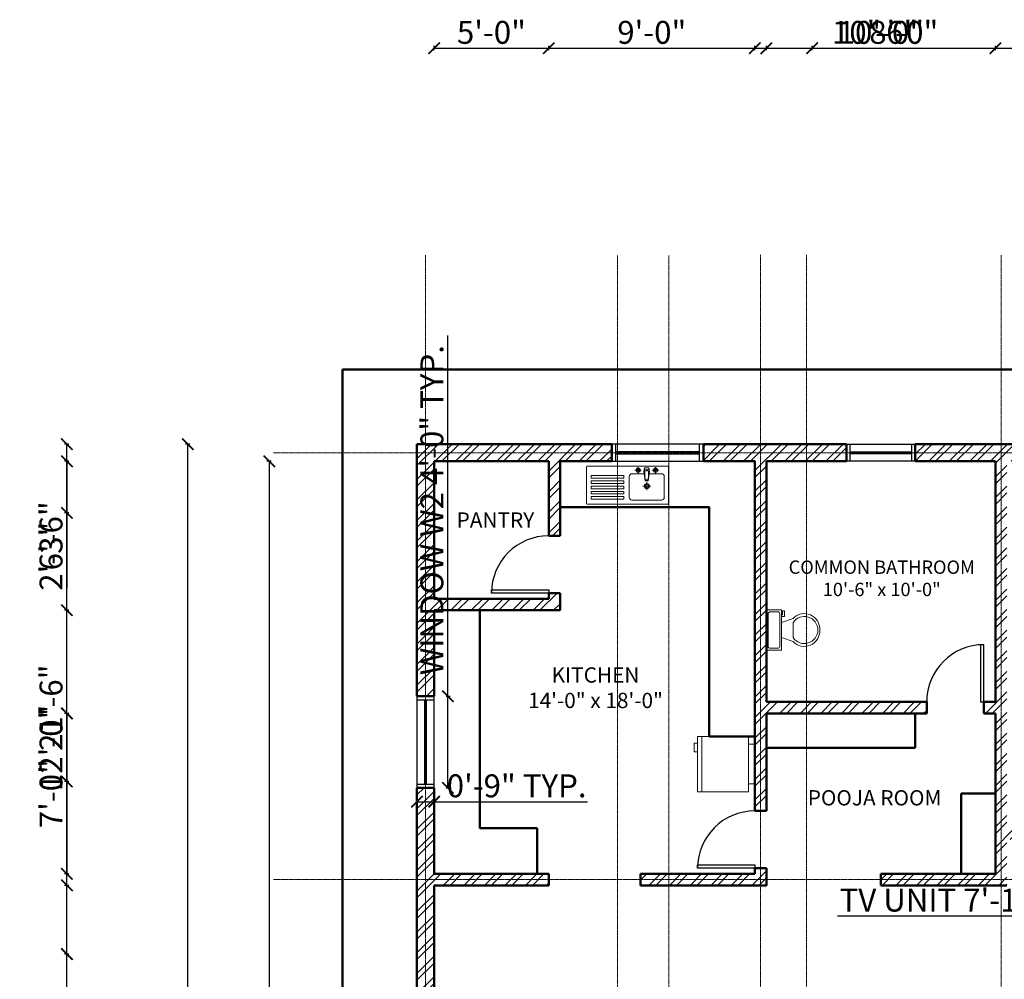
# Model space of a CAD drawing. Units: inches. Extents: x 261 to 2725, y 291 to 1454.
# Tile 13 of 35: x 261 to 777, y 951 to 1454. Entities that reach past the tile are written whole.
import ezdxf

# ---------------------------------------------------------------- set-up
doc = ezdxf.new("R2010")
doc.units = ezdxf.units.IN
doc.linetypes.add('CENTER', pattern=[2, 1.25, -0.25, 0.25, -0.25])
for name, color, linetype, lineweight in [('A-ANNO-DIMS', 136, 'Continuous', 18), ('A-AREA-IDEN', 18, 'Continuous', 18), ('A-DOOR', 160, 'Continuous', 25), ('A-FLOR-FIXT', 145, 'Continuous', 18), ('A-GLAZ', 150, 'Continuous', 25), ('A-GRID', 251, 'CENTER', 13), ('A-WALL', 222, 'Continuous', 50), ('A-WALL-PATT', 243, 'Continuous', 13)]:
    doc.layers.add(name, color=color, linetype=linetype, lineweight=lineweight)
doc.styles.get("Standard").update_dxf_attribs({"font": 'arial.ttf'})
doc.dimstyles.new('ISO-25', dxfattribs={"dimtxt": 12, "dimasz": 6, "dimexe": 1.25, "dimexo": 0.625, "dimtad": 1, "dimdec": 0, "dimlunit": 3, "dimtxsty": 'Standard', "dimblk": 'ARCHTICK', "dimcen": 2.5, "dimadec": 0, "dimazin": 0, "dimtfac": 1, "dimtdec": 0, "dimtmove": 0, "dimatfit": 3, "dimfxl": 1, "dimfxlon": 1, "dimarcsym": 0})

# ---------------------------------------------------------------- blocks, each defined once
blk = doc.blocks.new('*U3')
for p, q in [((0, 0), (0, -6)), ((30, 0), (30, -6))]:
    blk.add_line(p, q)
blk.add_lwpolyline([(0, 0), (0, 30), (1.75, 30), (1.75, 0)], close=True)
blk.add_arc((0, 0), 30, 0, 90)
blk = doc.blocks.new('*U4')
for p, q in [((-30, 0), (-30, -6)), ((0, 0), (0, -6))]:
    blk.add_line(p, q)
blk.add_lwpolyline([(0, 0), (0, 30), (-1.75, 30), (-1.75, 0)], close=True)
blk.add_arc((0, 0), 30, 90, 180)
blk = doc.blocks.new('A$C7C492201')
for p, q in [((0, 10), (0, 427)), ((10, 437), (927, 437)), ((221, 349), (78, 349)), ((112, 389), (185, 389)), ((148, 425), (148, 352)), ((223, 415), (217, 376)), ((217, 376), (232, 268)), ((223, 415), (232, 268)), ((223, 415), (248, 415)), ((225, 395), (248, 395)), ((273, 415), (248, 415)), ((272, 395), (248, 395)), ((273, 415), (265, 268)), ((280, 376), (265, 268)), ((273, 415), (280, 376)), ((418, 349), (276, 349)), ((312, 389), (385, 389)), ((348, 425), (348, 352)), ((937, 10), (937, 427)), ((48, 319), (48, 79)), ((231, 279), (248, 279)), ((232, 268), (248, 268)), ((266, 279), (248, 279)), ((265, 268), (248, 268)), ((248, 253), (248, 163)), ((448, 319), (448, 79)), ((509, 328), (509, 298)), ((509, 328), (885, 328)), ((509, 298), (885, 298)), ((509, 268), (509, 238)), ((509, 268), (885, 268)), ((509, 238), (885, 238)), ((885, 328), (885, 298)), ((885, 268), (885, 238)), ((203, 208), (294, 208)), ((509, 208), (885, 208)), ((509, 208), (509, 178)), ((509, 178), (885, 178)), ((509, 148), (509, 118)), ((509, 148), (885, 148)), ((509, 118), (885, 118)), ((885, 208), (885, 178)), ((885, 148), (885, 118)), ((927, 0), (10, 0)), ((418, 49), (78, 49)), ((509, 88), (509, 58)), ((509, 88), (885, 88)), ((509, 58), (885, 58)), ((885, 88), (885, 58))]:
    blk.add_line(p, q)
for centre, radius in [((148, 389), 25), ((148, 389), 15), ((348, 389), 25), ((348, 389), 15), ((248, 208), 30), ((248, 208), 20)]:
    blk.add_circle(centre, radius)
for centre, radius, start, end in [((10, 427), 10, 90, 180), ((78, 319), 30, 90, 180), ((247, 388), 7.19, 80.5252, 279.4748), ((250, 388), 7.19, 260.5252, 99.4748), ((418, 319), 30, 0, 90), ((927, 427), 10, 0, 90), ((10, 10), 10, 180, 270), ((78, 79), 30, 180, 270), ((418, 79), 30, 270, 0), ((927, 10), 10, 270, 0)]:
    blk.add_arc(centre, radius, start, end)
blk = doc.blocks.new('A$C659B0DF6')
for p, q in [((423, 642), (423, 606)), ((513, 642), (423, 642)), ((513, 606), (513, 642)), ((585, 606), (0, 606)), ((0, 66), (0, 606)), ((585, 561), (0, 561)), ((585, 66), (585, 606)), ((0, 66), (585, 66)), ((82, 0), (82, 66)), ((503, 0), (503, 66)), ((82, 0), (503, 0))]:
    blk.add_line(p, q)
blk = doc.blocks.new('*U27')
for p, q in [((9.5, -6), (9.5, -2)), ((-10, -8.5), (-8, -8.5)), ((-10, -9.5), (-10, -8.5)), ((-7, -9.5), (-10, -9.5)), ((-8, -8.5), (-8, -8)), ((-7, -8), (-7, -9.5)), ((-4, -8), (-6, -14)), ((4, -8), (6, -14)), ((4, -14), (-4, -14))]:
    blk.add_line(p, q)
blk.add_lwpolyline([(10.5, -8), (10.5, 0), (-10.5, 0), (-10.5, -8)], close=True)
for points in [[(-9.5, -2), (-9.5, -6)], [(8.5, -1), (-8.5, -1)], [(-8.5, -7), (8.5, -7)]]:
    blk.add_lwpolyline(points)
for centre, radius, start, end in [((-8.625, -1.875), 0.8839, 81.8699, 188.1301), ((8.625, -1.875), 0.8839, 351.8699, 98.1301), ((-8.625, -6.125), 0.8839, 171.869898, 278.1301), ((8.625, -6.125), 0.8839, 261.8699, 8.1301), ((-0.4772, -19.9188), 8.0953, 133.01722, 273.38), ((0.0374, -19.8731), 7.127, 124.50543, 269.7), ((-0.0373, -19.8731), 7.127, 270.3, 55.4946), ((0.4773, -19.9188), 8.0953, 266.62, 46.9828)]:
    blk.add_arc(centre, radius, start, end)
blk = doc.blocks.new('_ArchTick')
at = {"color": 0, "linetype": 'ByBlock', "const_width": 0.15}
blk.add_lwpolyline([(-0.5, -0.5), (0.5, 0.5)], dxfattribs=at)
blk = doc.blocks.new('*D29')
at = {"layer": 'A-ANNO-DIMS', "color": 0, "lineweight": -2, "transparency": 16777216}
for p, q in [((350.37, 1231.47), (348.12, 1231.47)), ((349.37, 508.47), (349.37, 1231.47)), ((350.37, 508.47), (348.12, 508.47))]:
    blk.add_line(p, q, dxfattribs=at)
at = {"layer": 'Defpoints', "color": 0, "transparency": 16777216}
for p in [(349.37, 1231.47), (469.45, 1231.47), (469.45, 508.47)]:
    blk.add_point(p, dxfattribs=at)
at = {"layer": 'A-ANNO-DIMS', "color": 0, "lineweight": -2, "transparency": 16777216, "xscale": 6, "yscale": 6, "zscale": 6}
for p, rotation in [((349.37, 1231.47), 90), ((349.37, 508.47), 270)]:
    blk.add_blockref('_ArchTick', p, dxfattribs=dict(at, rotation=rotation))
at = {"layer": 'A-ANNO-DIMS', "color": 0, "transparency": 16777216, "insert": (342.61, 869.97), "char_height": 12, "attachment_point": 5, "rotation": 90}
blk.add_mtext('60\'-3"', dxfattribs=at)
blk = doc.blocks.new('*D30')
at = {"layer": 'A-ANNO-DIMS', "color": 0, "lineweight": -2, "transparency": 16777216}
for p, q in [((393.09, 1222.47), (390.84, 1222.47)), ((392.09, 1222.47), (392.09, 517.47)), ((393.09, 517.47), (390.84, 517.47))]:
    blk.add_line(p, q, dxfattribs=at)
at = {"layer": 'Defpoints', "color": 0, "transparency": 16777216}
for p in [(478.45, 1222.47), (392.09, 517.47), (478.45, 517.47)]:
    blk.add_point(p, dxfattribs=at)
at = {"layer": 'A-ANNO-DIMS', "color": 0, "lineweight": -2, "transparency": 16777216, "xscale": 6, "yscale": 6, "zscale": 6}
for p, rotation in [((392.09, 1222.47), 90), ((392.09, 517.47), 270)]:
    blk.add_blockref('_ArchTick', p, dxfattribs=dict(at, rotation=rotation))
at = {"layer": 'A-ANNO-DIMS', "color": 0, "transparency": 16777216, "insert": (385.34, 869.97), "char_height": 12, "attachment_point": 5, "rotation": 90}
blk.add_mtext('58\'-9"', dxfattribs=at)
blk = doc.blocks.new('WIN-48')
for p, q in [((478.45, 1097.47), (469.45, 1097.47)), ((473.45, 1097.47), (473.45, 1053.47)), ((474.45, 1053.47), (474.45, 1097.47)), ((469.45, 1053.47), (478.45, 1053.47))]:
    blk.add_line(p, q)
blk.add_lwpolyline([(478.45, 1099.47), (469.45, 1099.47), (469.45, 1051.47), (478.45, 1051.47)], close=True)
blk = doc.blocks.new('WIN-36')
for p, q in [((1252.08, 755.47), (1243.08, 755.47)), ((1247.08, 755.47), (1247.08, 723.47)), ((1248.08, 723.47), (1248.08, 755.47)), ((1243.08, 723.47), (1252.08, 723.47))]:
    blk.add_line(p, q)
blk.add_lwpolyline([(1252.08, 721.47), (1252.08, 757.47), (1243.08, 757.47), (1243.08, 721.47)], close=True)
blk = doc.blocks.new('*D47')
at = {"layer": 'A-ANNO-DIMS', "color": 0, "lineweight": -2, "ltscale": 0.07, "transparency": 16777216}
for p, q in [((836.24, 985.34), (836.24, 983.09)), ((931.53, 985.34), (931.53, 983.09)), ((836.24, 984.34), (689.66, 984.34)), ((931.53, 984.34), (836.24, 984.34))]:
    blk.add_line(p, q, dxfattribs=at)
at = {"layer": 'Defpoints', "color": 0, "ltscale": 0.07, "transparency": 16777216}
for p in [(836.24, 998.63), (931.53, 998.63), (836.24, 984.34)]:
    blk.add_point(p, dxfattribs=at)
at = {"layer": 'A-ANNO-DIMS', "color": 0, "lineweight": -2, "ltscale": 0.07, "transparency": 16777216, "xscale": 6, "yscale": 6, "zscale": 6, "rotation": 180}
blk.add_blockref('_ArchTick', (836.24, 984.34), dxfattribs=at)
at = {"layer": 'A-ANNO-DIMS', "color": 0, "lineweight": -2, "ltscale": 0.07, "transparency": 16777216, "xscale": 6, "yscale": 6, "zscale": 6}
blk.add_blockref('_ArchTick', (931.53, 984.34), dxfattribs=at)
at = {"layer": 'A-ANNO-DIMS', "color": 0, "ltscale": 0.07, "transparency": 16777216, "insert": (759.95, 991.17), "char_height": 12, "attachment_point": 5}
blk.add_mtext('TV UNIT 7\'-11 1/2"', dxfattribs=at)
blk = doc.blocks.new('*D57')
at = {"layer": 'A-ANNO-DIMS', "color": 0, "lineweight": -2, "ltscale": 0.07, "transparency": 16777216}
for p, q in [((485.65, 1099.47), (485.65, 1288.37)), ((484.65, 1099.47), (486.9, 1099.47)), ((485.65, 1051.47), (485.65, 1099.47)), ((484.65, 1051.47), (486.9, 1051.47))]:
    blk.add_line(p, q, dxfattribs=at)
at = {"layer": 'Defpoints', "color": 0, "ltscale": 0.07, "transparency": 16777216}
for p in [(478.45, 1099.47), (485.65, 1099.47), (478.45, 1051.47)]:
    blk.add_point(p, dxfattribs=at)
at = {"layer": 'A-ANNO-DIMS', "color": 0, "lineweight": -2, "ltscale": 0.07, "transparency": 16777216, "xscale": 6, "yscale": 6, "zscale": 6}
for p, rotation in [((485.65, 1099.47), 90), ((485.65, 1051.47), 270)]:
    blk.add_blockref('_ArchTick', p, dxfattribs=dict(at, rotation=rotation))
at = {"layer": 'A-ANNO-DIMS', "color": 0, "ltscale": 0.07, "transparency": 16777216, "insert": (478.82, 1196.92), "char_height": 12, "attachment_point": 5, "rotation": 90}
blk.add_mtext('WINDOW W2 4\'-0" TYP.', dxfattribs=at)
blk = doc.blocks.new('*D58')
at = {"layer": 'A-ANNO-DIMS', "color": 0, "lineweight": -2, "ltscale": 0.07, "transparency": 16777216}
for p, q in [((469.45, 1045.27), (469.45, 1043.02)), ((469.45, 1044.27), (478.45, 1044.27)), ((478.45, 1045.27), (478.45, 1043.02)), ((478.45, 1044.27), (558.85, 1044.27))]:
    blk.add_line(p, q, dxfattribs=at)
at = {"layer": 'Defpoints', "color": 0, "ltscale": 0.07, "transparency": 16777216}
for p in [(469.45, 1051.47), (478.45, 1051.47), (478.45, 1044.27)]:
    blk.add_point(p, dxfattribs=at)
at = {"layer": 'A-ANNO-DIMS', "color": 0, "lineweight": -2, "ltscale": 0.07, "transparency": 16777216, "xscale": 6, "yscale": 6, "zscale": 6, "rotation": 180}
blk.add_blockref('_ArchTick', (469.45, 1044.27), dxfattribs=at)
at = {"layer": 'A-ANNO-DIMS', "color": 0, "lineweight": -2, "ltscale": 0.07, "transparency": 16777216, "xscale": 6, "yscale": 6, "zscale": 6}
blk.add_blockref('_ArchTick', (478.45, 1044.27), dxfattribs=at)
at = {"layer": 'A-ANNO-DIMS', "color": 0, "ltscale": 0.07, "transparency": 16777216, "insert": (521.65, 1051.02), "char_height": 12, "attachment_point": 5}
blk.add_mtext('0\'-9" TYP.', dxfattribs=at)
blk = doc.blocks.new('*D73')
at = {"layer": 'A-ANNO-DIMS', "color": 0, "lineweight": -2, "ltscale": 0.07, "transparency": 16777216}
for p, q in [((478.45, 1437.76), (478.45, 1440.01)), ((538.45, 1437.76), (538.45, 1440.01)), ((478.45, 1438.76), (538.45, 1438.76))]:
    blk.add_line(p, q, dxfattribs=at)
at = {"layer": 'Defpoints', "color": 0, "ltscale": 0.07, "transparency": 16777216}
for p in [(538.45, 1438.76), (478.45, 1222.47), (538.45, 1222.47)]:
    blk.add_point(p, dxfattribs=at)
at = {"layer": 'A-ANNO-DIMS', "color": 0, "lineweight": -2, "ltscale": 0.07, "transparency": 16777216, "xscale": 6, "yscale": 6, "zscale": 6, "rotation": 180}
blk.add_blockref('_ArchTick', (478.45, 1438.76), dxfattribs=at)
at = {"layer": 'A-ANNO-DIMS', "color": 0, "lineweight": -2, "ltscale": 0.07, "transparency": 16777216, "xscale": 6, "yscale": 6, "zscale": 6}
blk.add_blockref('_ArchTick', (538.45, 1438.76), dxfattribs=at)
at = {"layer": 'A-ANNO-DIMS', "color": 0, "ltscale": 0.07, "transparency": 16777216, "insert": (508.45, 1445.51), "char_height": 12, "attachment_point": 5}
blk.add_mtext('5\'-0"', dxfattribs=at)
blk = doc.blocks.new('*D74')
at = {"layer": 'A-ANNO-DIMS', "color": 0, "lineweight": -2, "ltscale": 0.07, "transparency": 16777216}
for p, q in [((538.45, 1437.76), (538.45, 1440.01)), ((646.45, 1437.76), (646.45, 1440.01)), ((538.45, 1438.76), (646.45, 1438.76))]:
    blk.add_line(p, q, dxfattribs=at)
at = {"layer": 'Defpoints', "color": 0, "ltscale": 0.07, "transparency": 16777216}
for p in [(646.45, 1438.76), (538.45, 1222.47), (646.45, 1222.47)]:
    blk.add_point(p, dxfattribs=at)
at = {"layer": 'A-ANNO-DIMS', "color": 0, "lineweight": -2, "ltscale": 0.07, "transparency": 16777216, "xscale": 6, "yscale": 6, "zscale": 6, "rotation": 180}
blk.add_blockref('_ArchTick', (538.45, 1438.76), dxfattribs=at)
at = {"layer": 'A-ANNO-DIMS', "color": 0, "lineweight": -2, "ltscale": 0.07, "transparency": 16777216, "xscale": 6, "yscale": 6, "zscale": 6}
blk.add_blockref('_ArchTick', (646.45, 1438.76), dxfattribs=at)
at = {"layer": 'A-ANNO-DIMS', "color": 0, "ltscale": 0.07, "transparency": 16777216, "insert": (592.45, 1445.51), "char_height": 12, "attachment_point": 5}
blk.add_mtext('9\'-0"', dxfattribs=at)
blk = doc.blocks.new('*D75')
at = {"layer": 'A-ANNO-DIMS', "color": 0, "lineweight": -2, "ltscale": 0.07, "transparency": 16777216}
for p, q in [((646.45, 1437.76), (646.45, 1440.01)), ((772.45, 1437.76), (772.45, 1440.01)), ((646.45, 1438.76), (772.45, 1438.76))]:
    blk.add_line(p, q, dxfattribs=at)
at = {"layer": 'Defpoints', "color": 0, "ltscale": 0.07, "transparency": 16777216}
for p in [(772.45, 1438.76), (646.45, 1222.47), (772.45, 1222.47)]:
    blk.add_point(p, dxfattribs=at)
at = {"layer": 'A-ANNO-DIMS', "color": 0, "lineweight": -2, "ltscale": 0.07, "transparency": 16777216, "xscale": 6, "yscale": 6, "zscale": 6, "rotation": 180}
blk.add_blockref('_ArchTick', (646.45, 1438.76), dxfattribs=at)
at = {"layer": 'A-ANNO-DIMS', "color": 0, "lineweight": -2, "ltscale": 0.07, "transparency": 16777216, "xscale": 6, "yscale": 6, "zscale": 6}
blk.add_blockref('_ArchTick', (772.45, 1438.76), dxfattribs=at)
at = {"layer": 'A-ANNO-DIMS', "color": 0, "ltscale": 0.07, "transparency": 16777216, "insert": (709.45, 1445.51), "char_height": 12, "attachment_point": 5}
blk.add_mtext('10\'-6"', dxfattribs=at)
blk = doc.blocks.new('*D76')
at = {"layer": 'A-ANNO-DIMS', "color": 0, "lineweight": -2, "ltscale": 0.07, "transparency": 16777216}
for p, q in [((772.45, 1437.76), (772.45, 1440.01)), ((946.45, 1437.76), (946.45, 1440.01)), ((772.45, 1438.76), (946.45, 1438.76))]:
    blk.add_line(p, q, dxfattribs=at)
at = {"layer": 'Defpoints', "color": 0, "ltscale": 0.07, "transparency": 16777216}
for p in [(946.45, 1438.76), (772.45, 1222.47), (946.45, 1222.47)]:
    blk.add_point(p, dxfattribs=at)
at = {"layer": 'A-ANNO-DIMS', "color": 0, "lineweight": -2, "ltscale": 0.07, "transparency": 16777216, "xscale": 6, "yscale": 6, "zscale": 6, "rotation": 180}
blk.add_blockref('_ArchTick', (772.45, 1438.76), dxfattribs=at)
at = {"layer": 'A-ANNO-DIMS', "color": 0, "lineweight": -2, "ltscale": 0.07, "transparency": 16777216, "xscale": 6, "yscale": 6, "zscale": 6}
blk.add_blockref('_ArchTick', (946.45, 1438.76), dxfattribs=at)
at = {"layer": 'A-ANNO-DIMS', "color": 0, "ltscale": 0.07, "transparency": 16777216, "insert": (859.45, 1445.51), "char_height": 12, "attachment_point": 5}
blk.add_mtext('14\'-6"', dxfattribs=at)
blk = doc.blocks.new('*D79')
at = {"layer": 'A-ANNO-DIMS', "color": 0, "lineweight": -2, "ltscale": 0.07, "transparency": 16777216}
for p, q in [((287.06, 1000.47), (284.81, 1000.47)), ((286.06, 784.47), (286.06, 1000.47)), ((287.06, 784.47), (284.81, 784.47))]:
    blk.add_line(p, q, dxfattribs=at)
at = {"layer": 'Defpoints', "color": 0, "ltscale": 0.07, "transparency": 16777216}
for p in [(286.06, 1000.47), (478.45, 1000.47), (478.45, 784.47)]:
    blk.add_point(p, dxfattribs=at)
at = {"layer": 'A-ANNO-DIMS', "color": 0, "lineweight": -2, "ltscale": 0.07, "transparency": 16777216, "xscale": 6, "yscale": 6, "zscale": 6}
for p, rotation in [((286.06, 1000.47), 90), ((286.06, 784.47), 270)]:
    blk.add_blockref('_ArchTick', p, dxfattribs=dict(at, rotation=rotation))
at = {"layer": 'A-ANNO-DIMS', "color": 0, "ltscale": 0.07, "transparency": 16777216, "insert": (279.3, 892.47), "char_height": 12, "attachment_point": 5, "rotation": 90}
blk.add_mtext('18\'-0"', dxfattribs=at)
blk = doc.blocks.new('*D80')
at = {"layer": 'A-ANNO-DIMS', "color": 0, "lineweight": -2, "ltscale": 0.07, "transparency": 16777216}
for p, q in [((287.06, 1144.47), (284.81, 1144.47)), ((286.06, 1000.47), (286.06, 1144.47)), ((287.06, 1000.47), (284.81, 1000.47))]:
    blk.add_line(p, q, dxfattribs=at)
at = {"layer": 'Defpoints', "color": 0, "ltscale": 0.07, "transparency": 16777216}
for p in [(286.06, 1144.47), (478.45, 1144.47), (478.45, 1000.47)]:
    blk.add_point(p, dxfattribs=at)
at = {"layer": 'A-ANNO-DIMS', "color": 0, "lineweight": -2, "ltscale": 0.07, "transparency": 16777216, "xscale": 6, "yscale": 6, "zscale": 6}
for p, rotation in [((286.06, 1144.47), 90), ((286.06, 1000.47), 270)]:
    blk.add_blockref('_ArchTick', p, dxfattribs=dict(at, rotation=rotation))
at = {"layer": 'A-ANNO-DIMS', "color": 0, "ltscale": 0.07, "transparency": 16777216, "insert": (279.3, 1072.47), "char_height": 12, "attachment_point": 5, "rotation": 90}
blk.add_mtext('12\'-0"', dxfattribs=at)
blk = doc.blocks.new('*D81')
at = {"layer": 'A-ANNO-DIMS', "color": 0, "lineweight": -2, "ltscale": 0.07, "transparency": 16777216}
for p, q in [((287.06, 1222.47), (284.81, 1222.47)), ((286.06, 1144.47), (286.06, 1222.47)), ((287.06, 1144.47), (284.81, 1144.47))]:
    blk.add_line(p, q, dxfattribs=at)
at = {"layer": 'Defpoints', "color": 0, "ltscale": 0.07, "transparency": 16777216}
for p in [(286.06, 1222.47), (478.45, 1222.47), (478.45, 1144.47)]:
    blk.add_point(p, dxfattribs=at)
at = {"layer": 'A-ANNO-DIMS', "color": 0, "lineweight": -2, "ltscale": 0.07, "transparency": 16777216, "xscale": 6, "yscale": 6, "zscale": 6}
for p, rotation in [((286.06, 1222.47), 90), ((286.06, 1144.47), 270)]:
    blk.add_blockref('_ArchTick', p, dxfattribs=dict(at, rotation=rotation))
at = {"layer": 'A-ANNO-DIMS', "color": 0, "ltscale": 0.07, "transparency": 16777216, "insert": (279.3, 1183.47), "char_height": 12, "attachment_point": 5, "rotation": 90}
blk.add_mtext('6\'-6"', dxfattribs=at)
blk = doc.blocks.new('*D86')
at = {"layer": 'A-ANNO-DIMS', "color": 0, "lineweight": -2, "ltscale": 0.07, "transparency": 16777216}
for p, q in [((676.45, 1437.76), (676.45, 1440.01)), ((772.45, 1437.76), (772.45, 1440.01)), ((676.45, 1438.76), (772.45, 1438.76))]:
    blk.add_line(p, q, dxfattribs=at)
at = {"layer": 'Defpoints', "color": 0, "ltscale": 0.07, "transparency": 16777216}
for p in [(772.45, 1438.76), (676.45, 517.47), (772.45, 517.47)]:
    blk.add_point(p, dxfattribs=at)
at = {"layer": 'A-ANNO-DIMS', "color": 0, "lineweight": -2, "ltscale": 0.07, "transparency": 16777216, "xscale": 6, "yscale": 6, "zscale": 6, "rotation": 180}
blk.add_blockref('_ArchTick', (676.45, 1438.76), dxfattribs=at)
at = {"layer": 'A-ANNO-DIMS', "color": 0, "lineweight": -2, "ltscale": 0.07, "transparency": 16777216, "xscale": 6, "yscale": 6, "zscale": 6}
blk.add_blockref('_ArchTick', (772.45, 1438.76), dxfattribs=at)
at = {"layer": 'A-ANNO-DIMS', "color": 0, "ltscale": 0.07, "transparency": 16777216, "insert": (724.45, 1445.51), "char_height": 12, "attachment_point": 5}
blk.add_mtext('8\'-0"', dxfattribs=at)
blk = doc.blocks.new('*D94')
at = {"layer": 'A-ANNO-DIMS', "color": 0, "lineweight": -2, "ltscale": 0.07, "transparency": 16777216}
for p, q in [((652.45, 1437.76), (652.45, 1440.01)), ((772.45, 1437.76), (772.45, 1440.01)), ((652.45, 1438.76), (772.45, 1438.76))]:
    blk.add_line(p, q, dxfattribs=at)
at = {"layer": 'Defpoints', "color": 0, "ltscale": 0.07, "transparency": 16777216}
for p in [(772.45, 1438.76), (652.45, 1090.47), (772.45, 1090.47)]:
    blk.add_point(p, dxfattribs=at)
at = {"layer": 'A-ANNO-DIMS', "color": 0, "lineweight": -2, "ltscale": 0.07, "transparency": 16777216, "xscale": 6, "yscale": 6, "zscale": 6, "rotation": 180}
blk.add_blockref('_ArchTick', (652.45, 1438.76), dxfattribs=at)
at = {"layer": 'A-ANNO-DIMS', "color": 0, "lineweight": -2, "ltscale": 0.07, "transparency": 16777216, "xscale": 6, "yscale": 6, "zscale": 6}
blk.add_blockref('_ArchTick', (772.45, 1438.76), dxfattribs=at)
at = {"layer": 'A-ANNO-DIMS', "color": 0, "ltscale": 0.07, "transparency": 16777216, "insert": (712.45, 1445.51), "char_height": 12, "attachment_point": 5}
blk.add_mtext('10\'-0"', dxfattribs=at)
blk = doc.blocks.new('*D95')
at = {"layer": 'A-ANNO-DIMS', "color": 0, "lineweight": -2, "ltscale": 0.07, "transparency": 16777216}
for p, q in [((287.06, 1090.47), (284.81, 1090.47)), ((286.06, 1090.47), (286.06, 1006.47)), ((287.06, 1006.47), (284.81, 1006.47))]:
    blk.add_line(p, q, dxfattribs=at)
at = {"layer": 'Defpoints', "color": 0, "ltscale": 0.07, "transparency": 16777216}
for p in [(652.45, 1090.47), (286.06, 1006.47), (712.45, 1006.47)]:
    blk.add_point(p, dxfattribs=at)
at = {"layer": 'A-ANNO-DIMS', "color": 0, "lineweight": -2, "ltscale": 0.07, "transparency": 16777216, "xscale": 6, "yscale": 6, "zscale": 6}
for p, rotation in [((286.06, 1090.47), 90), ((286.06, 1006.47), 270)]:
    blk.add_blockref('_ArchTick', p, dxfattribs=dict(at, rotation=rotation))
at = {"layer": 'A-ANNO-DIMS', "color": 0, "ltscale": 0.07, "transparency": 16777216, "insert": (279.3, 1048.47), "char_height": 12, "attachment_point": 5, "rotation": 90}
blk.add_mtext('7\'-0"', dxfattribs=at)
blk = doc.blocks.new('*D103')
at = {"layer": 'A-ANNO-DIMS', "color": 0, "lineweight": -2, "ltscale": 0.07, "transparency": 16777216}
for p, q in [((287.06, 1231.47), (284.81, 1231.47)), ((286.06, 439.47), (286.06, 1231.47)), ((287.06, 439.47), (284.81, 439.47))]:
    blk.add_line(p, q, dxfattribs=at)
at = {"layer": 'Defpoints', "color": 0, "ltscale": 0.07, "transparency": 16777216}
for p in [(286.06, 1231.47), (1243.08, 1231.47), (1243.08, 439.47)]:
    blk.add_point(p, dxfattribs=at)
at = {"layer": 'A-ANNO-DIMS', "color": 0, "lineweight": -2, "ltscale": 0.07, "transparency": 16777216, "xscale": 6, "yscale": 6, "zscale": 6}
for p, rotation in [((286.06, 1231.47), 90), ((286.06, 439.47), 270)]:
    blk.add_blockref('_ArchTick', p, dxfattribs=dict(at, rotation=rotation))
at = {"layer": 'A-ANNO-DIMS', "color": 0, "ltscale": 0.07, "transparency": 16777216, "insert": (279.3, 835.47), "char_height": 12, "attachment_point": 5, "rotation": 90}
blk.add_mtext('66\'-0"', dxfattribs=at)
blk = doc.blocks.new('*D109')
at = {"layer": 'A-ANNO-DIMS', "color": 0, "lineweight": -2, "ltscale": 0.07, "transparency": 16777216}
for p, q in [((287.06, 964.47), (284.81, 964.47)), ((286.06, 799.47), (286.06, 964.47)), ((287.06, 799.47), (284.81, 799.47))]:
    blk.add_line(p, q, dxfattribs=at)
at = {"layer": 'Defpoints', "color": 0, "ltscale": 0.07, "transparency": 16777216}
for p in [(286.06, 964.47), (1252.08, 964.47), (1252.08, 799.47)]:
    blk.add_point(p, dxfattribs=at)
at = {"layer": 'A-ANNO-DIMS', "color": 0, "lineweight": -2, "ltscale": 0.07, "transparency": 16777216, "xscale": 6, "yscale": 6, "zscale": 6}
for p, rotation in [((286.06, 964.47), 90), ((286.06, 799.47), 270)]:
    blk.add_blockref('_ArchTick', p, dxfattribs=dict(at, rotation=rotation))
at = {"layer": 'A-ANNO-DIMS', "color": 0, "ltscale": 0.07, "transparency": 16777216, "insert": (279.3, 881.97), "char_height": 12, "attachment_point": 5, "rotation": 90}
blk.add_mtext('13\'-9"', dxfattribs=at)
blk = doc.blocks.new('*D110')
at = {"layer": 'A-ANNO-DIMS', "color": 0, "lineweight": -2, "ltscale": 0.07, "transparency": 16777216}
for p, q in [((287.06, 1222.47), (284.81, 1222.47)), ((286.06, 964.47), (286.06, 1222.47)), ((287.06, 964.47), (284.81, 964.47))]:
    blk.add_line(p, q, dxfattribs=at)
at = {"layer": 'Defpoints', "color": 0, "ltscale": 0.07, "transparency": 16777216}
for p in [(286.06, 1222.47), (1252.08, 1222.47), (1252.08, 964.47)]:
    blk.add_point(p, dxfattribs=at)
at = {"layer": 'A-ANNO-DIMS', "color": 0, "lineweight": -2, "ltscale": 0.07, "transparency": 16777216, "xscale": 6, "yscale": 6, "zscale": 6}
for p, rotation in [((286.06, 1222.47), 90), ((286.06, 964.47), 270)]:
    blk.add_blockref('_ArchTick', p, dxfattribs=dict(at, rotation=rotation))
at = {"layer": 'A-ANNO-DIMS', "color": 0, "ltscale": 0.07, "transparency": 16777216, "insert": (279.3, 1093.47), "char_height": 12, "attachment_point": 5, "rotation": 90}
blk.add_mtext('21\'-6"', dxfattribs=at)
blk = doc.blocks.new('*D118')
at = {"layer": 'A-ANNO-DIMS', "color": 0, "lineweight": -2, "ltscale": 0.07, "transparency": 16777216}
for p, q in [((287.06, 1222.47), (284.81, 1222.47)), ((286.06, 1222.47), (286.06, 1195.47)), ((287.06, 1195.47), (284.81, 1195.47)), ((286.06, 1195.47), (286.06, 1156.11))]:
    blk.add_line(p, q, dxfattribs=at)
at = {"layer": 'Defpoints', "color": 0, "ltscale": 0.07, "transparency": 16777216}
for p in [(1252.08, 1222.47), (286.06, 1195.47), (1252.08, 1195.47)]:
    blk.add_point(p, dxfattribs=at)
at = {"layer": 'A-ANNO-DIMS', "color": 0, "lineweight": -2, "ltscale": 0.07, "transparency": 16777216, "xscale": 6, "yscale": 6, "zscale": 6}
for p, rotation in [((286.06, 1222.47), 90), ((286.06, 1195.47), 270)]:
    blk.add_blockref('_ArchTick', p, dxfattribs=dict(at, rotation=rotation))
at = {"layer": 'A-ANNO-DIMS', "color": 0, "ltscale": 0.07, "transparency": 16777216, "insert": (279.3, 1172.79), "char_height": 12, "attachment_point": 5, "rotation": 90}
blk.add_mtext('2\'-3"', dxfattribs=at)
blk = doc.blocks.new('*D123')
at = {"layer": 'A-ANNO-DIMS', "color": 0, "lineweight": -2, "ltscale": 0.07, "transparency": 16777216}
for p, q in [((287.06, 1054.85), (284.81, 1054.85)), ((286.06, 439.47), (286.06, 1054.85)), ((287.06, 439.47), (284.81, 439.47))]:
    blk.add_line(p, q, dxfattribs=at)
at = {"layer": 'Defpoints', "color": 0, "ltscale": 0.07, "transparency": 16777216}
for p in [(286.06, 1054.85), (2007.71, 1054.85), (2007.71, 439.47)]:
    blk.add_point(p, dxfattribs=at)
at = {"layer": 'A-ANNO-DIMS', "color": 0, "lineweight": -2, "ltscale": 0.07, "transparency": 16777216, "xscale": 6, "yscale": 6, "zscale": 6}
for p, rotation in [((286.06, 1054.85), 90), ((286.06, 439.47), 270)]:
    blk.add_blockref('_ArchTick', p, dxfattribs=dict(at, rotation=rotation))
at = {"layer": 'A-ANNO-DIMS', "color": 0, "ltscale": 0.07, "transparency": 16777216, "insert": (279.22, 747.16), "char_height": 12, "attachment_point": 5, "rotation": 90}
blk.add_mtext('51\'-3 1/2"', dxfattribs=at)

msp = doc.modelspace()

# ---------------------------------------------------------------- hatches: boundary and pattern name
at = {"layer": 'A-WALL-PATT'}
h = msp.add_hatch(dxfattribs=at)
h.set_pattern_fill('ANSI32', color=256, scale=0.8)
h.paths.add_polyline_path([(478.45, 685.47), (580.45, 685.47), (580.45, 691.47), (577.45, 691.47), (577.45, 694.47), (571.45, 694.47), (571.45, 691.47), (478.45, 691.47), (478.45, 721.47), (469.45, 721.47), (469.45, 508.47), (538.45, 508.47), (538.45, 517.47), (478.45, 517.47)])
h.paths.add_polyline_path([(694.45, 517.47), (676.45, 517.47), (676.45, 646.47), (670.45, 646.47), (670.45, 517.47), (610.45, 517.47), (610.45, 508.47), (694.45, 508.47)])
h.paths.add_polyline_path([(676.45, 784.47), (478.45, 784.47), (478.45, 844.47), (469.45, 844.47), (469.45, 745.47), (478.45, 745.47), (478.45, 775.47), (571.45, 775.47), (571.45, 724.47), (577.45, 724.47), (577.45, 775.47), (670.45, 775.47), (670.45, 691.47), (610.45, 691.47), (610.45, 685.47), (670.45, 685.47), (670.45, 682.47), (676.45, 682.47)])
h.paths.add_polyline_path([(955.45, 880.47), (946.45, 880.47), (946.45, 808.47), (778.45, 808.47), (778.45, 799.47), (946.45, 799.47), (946.45, 517.47), (898.45, 517.47), (898.45, 508.47), (955.45, 508.47)])
h.paths.add_polyline_path([(778.45, 598.47), (772.45, 598.47), (772.45, 517.47), (754.45, 517.47), (754.45, 508.47), (826.45, 508.47), (826.45, 517.47), (778.45, 517.47)])
h.paths.add_polyline_path([(955.45, 1090.47), (946.45, 1090.47), (946.45, 1030.47), (817.45, 1030.47), (817.45, 1024.47), (946.45, 1024.47), (946.45, 952.47), (955.45, 952.47)])
h.paths.add_polyline_path([(955.45, 1231.47), (730.45, 1231.47), (730.45, 1222.47), (772.45, 1222.47), (772.45, 1096.47), (766.45, 1096.47), (766.45, 1090.47), (772.45, 1090.47), (772.45, 1006.47), (712.45, 1006.47), (712.45, 1000.47), (778.45, 1000.47), (778.45, 1024.47), (781.45, 1024.47), (781.45, 1030.47), (778.45, 1030.47), (778.45, 1222.47), (946.45, 1222.47), (946.45, 1162.47), (955.45, 1162.47)])
h.paths.add_polyline_path([(694.45, 1231.47), (619.45, 1231.47), (619.45, 1222.47), (646.45, 1222.47), (646.45, 1039.47), (652.45, 1039.47), (652.45, 1090.47), (736.45, 1090.47), (736.45, 1096.47), (652.45, 1096.47), (652.45, 1222.47), (694.45, 1222.47)])
h.paths.add_polyline_path([(571.45, 1231.47), (469.45, 1231.47), (469.45, 1099.47), (478.45, 1099.47), (478.45, 1144.47), (544.45, 1144.47), (544.45, 1153.47), (538.45, 1153.47), (538.45, 1150.47), (478.45, 1150.47), (478.45, 1222.47), (538.45, 1222.47), (538.45, 1183.47), (544.45, 1183.47), (544.45, 1222.47), (571.45, 1222.47)])
h.paths.add_polyline_path([(538.45, 1006.47), (478.45, 1006.47), (478.45, 1051.47), (469.45, 1051.47), (469.45, 940.47), (478.45, 940.47), (478.45, 1000.47), (538.45, 1000.47)])
h.paths.add_polyline_path([(652.45, 1006.47), (652.45, 1009.47), (646.45, 1009.47), (646.45, 1006.47), (586.45, 1006.47), (586.45, 1000.47), (652.45, 1000.47)])
h.paths.add_polyline_path([(1288.08, 973.47), (1243.08, 973.47), (1243.08, 920.97), (1252.08, 920.97), (1252.08, 964.47), (1288.08, 964.47)], flags=17)
h.paths.add_polyline_path([(1402.08, 805.47), (1252.08, 805.47), (1252.08, 848.97), (1243.08, 848.97), (1243.08, 757.47), (1252.08, 757.47), (1252.08, 799.47), (1294.08, 799.47), (1372.08, 799.47), (1372.08, 779.47), (1372.08, 715.47), (1378.08, 715.47), (1378.08, 799.47), (1402.08, 799.47)])
h.paths.add_polyline_path([(1252.08, 721.47), (1243.08, 721.47), (1243.08, 439.47), (1729.08, 439.47), (1729.08, 709.47), (1720.08, 709.47), (1720.08, 679.47), (1582.08, 679.47), (1582.08, 670.47), (1588.08, 670.47), (1588.08, 673.47), (1720.08, 673.47), (1720.08, 559.47), (1690.08, 559.47), (1690.08, 550.47), (1720.08, 550.47), (1720.08, 448.47), (1252.08, 448.47), (1252.08, 496.47), (1312.08, 496.47), (1312.08, 505.47), (1252.08, 505.47), (1252.08, 673.47), (1405.08, 673.47), (1405.08, 679.47), (1378.08, 679.47), (1378.08, 685.47), (1372.08, 685.47), (1372.08, 679.47), (1252.08, 679.47)])
h.paths.add_polyline_path([(1450.08, 550.47), (1480.08, 550.47), (1480.08, 559.47), (1450.08, 559.47), (1450.08, 679.47), (1441.08, 679.47), (1441.08, 673.47), (1444.08, 673.47), (1444.08, 505.47), (1384.08, 505.47), (1384.08, 496.47), (1450.08, 496.47)], flags=17)
h.paths.add_polyline_path([(1618.08, 559.47), (1588.08, 559.47), (1588.08, 634.47), (1582.08, 634.47), (1582.08, 559.47), (1552.08, 559.47), (1552.08, 550.47), (1618.08, 550.47)], flags=17)
h.paths.add_polyline_path([(1564.08, 964.47), (1630.08, 964.47), (1630.08, 973.47), (1477.08, 973.47), (1477.08, 964.47), (1558.08, 964.47), (1558.08, 926.22), (1558.08, 887.97), (1486.08, 887.97), (1486.08, 881.97), (1558.08, 881.97), (1558.08, 805.47), (1450.08, 805.47), (1450.08, 845.97), (1444.08, 845.97), (1444.08, 805.47), (1438.08, 805.47), (1438.08, 799.47), (1564.08, 799.47)], flags=17)
h.paths.add_polyline_path([(1453.08, 973.47), (1408.08, 973.47), (1408.08, 964.47), (1444.08, 964.47), (1444.08, 881.97), (1450.08, 881.97), (1456.08, 881.97), (1456.08, 887.97), (1450.08, 887.97), (1450.08, 964.47), (1453.08, 964.47)], flags=17)
h.paths.add_polyline_path([(1729.08, 1231.47), (1243.08, 1231.47), (1243.08, 1167.47), (1252.08, 1167.47), (1252.08, 1222.47), (1441.08, 1222.47), (1441.08, 1045.47), (1648.08, 1045.47), (1648.08, 1051.47), (1450.08, 1051.47), (1450.08, 1074.47), (1450.08, 1222.47), (1472.08, 1222.47), (1720.08, 1222.47), (1720.08, 1051.47), (1708.08, 1051.47), (1708.08, 1045.47), (1720.08, 1045.47), (1720.08, 973.47), (1702.08, 973.47), (1702.08, 964.47), (1720.08, 964.47), (1720.08, 769.47), (1729.08, 769.47)])
h.paths.add_polyline_path([(2493.71, 1054.85), (2007.71, 1054.85), (2007.71, 439.47), (2214.67, 439.47), (2214.67, 496.47), (2493.71, 496.47)])
h.paths.add_polyline_path([(2016.71, 1045.85), (2304.71, 1045.85), (2304.71, 841.47), (2310.71, 841.47), (2310.71, 1045.85), (2484.71, 1045.85), (2484.71, 805.47), (2310.71, 805.47), (2310.71, 811.47), (2304.71, 811.47), (2304.71, 799.47), (2484.71, 799.47), (2484.71, 679.47), (2304.71, 679.47), (2304.71, 673.47), (2484.71, 673.47), (2484.71, 505.47), (2208.67, 505.47), (2208.67, 448.47), (2016.71, 448.47), (2016.71, 799.47), (2304.71, 799.47), (2304.71, 805.47), (2016.71, 805.47)], flags=16)

# ---------------------------------------------------------------- linework, layer by layer
at = {"layer": 'A-GRID', "ltscale": 0.5}
for p, q in [((473.95, 1330.47), (473.95, 416.47)), ((574.45, 1330.18), (574.45, 416.18)), ((601.45, 1330.18), (601.45, 416.18)), ((649.45, 1330.51), (649.45, 416.51)), ((673.45, 1330.51), (673.45, 416.51)), ((775.45, 1330.47), (775.45, 416.47)), ((394.31, 1226.97), (1018.31, 1226.97)), ((394.31, 1003.47), (1018.31, 1003.47))]:
    msp.add_line(p, q, dxfattribs=at)
at = {"layer": 'A-WALL'}
for p, q in [((430.45, 1270.47), (430.45, 412.47)), ((994.45, 1270.47), (430.45, 1270.47)), ((469.45, 1231.47), (469.45, 1099.47)), ((571.45, 1231.47), (469.45, 1231.47)), ((571.45, 1222.47), (571.45, 1231.47)), ((619.45, 1222.47), (619.45, 1231.47)), ((694.45, 1231.47), (619.45, 1231.47)), ((694.45, 1222.47), (694.45, 1231.47)), ((955.45, 1231.47), (730.45, 1231.47)), ((730.45, 1222.47), (730.45, 1231.47)), ((478.45, 1222.47), (478.45, 1150.47)), ((538.45, 1222.47), (478.45, 1222.47)), ((538.45, 1222.47), (538.45, 1183.47)), ((544.45, 1222.47), (544.45, 1183.47)), ((571.45, 1222.47), (544.45, 1222.47)), ((652.45, 1222.47), (652.45, 1096.47)), ((694.45, 1222.47), (652.45, 1222.47)), ((772.45, 1222.47), (730.45, 1222.47)), ((772.45, 1222.47), (772.45, 1096.47)), ((538.45, 1183.47), (544.45, 1183.47)), ((538.45, 1150.47), (478.45, 1150.47)), ((538.45, 1153.47), (544.45, 1153.47)), ((538.45, 1153.47), (538.45, 1150.47)), ((544.45, 1153.47), (544.45, 1144.47)), ((544.45, 1144.47), (478.45, 1144.47)), ((478.45, 1144.47), (478.45, 1099.47)), ((478.45, 1099.47), (469.45, 1099.47)), ((736.45, 1096.47), (652.45, 1096.47)), ((736.45, 1090.47), (736.45, 1096.47)), ((772.45, 1096.47), (766.45, 1096.47)), ((766.45, 1090.47), (766.45, 1096.47)), ((652.45, 1090.47), (652.45, 1039.47)), ((736.45, 1090.47), (652.45, 1090.47)), ((730.45, 1090.47), (730.45, 1072.47)), ((772.45, 1090.47), (766.45, 1090.47)), ((772.45, 1090.47), (772.45, 1006.47)), ((622.45, 1078.47), (646.45, 1078.47)), ((730.45, 1072.47), (652.45, 1072.47)), ((478.45, 1051.47), (469.45, 1051.47)), ((469.45, 1051.47), (469.45, 940.47)), ((754.45, 1048.47), (754.45, 1006.47)), ((772.45, 1048.47), (754.45, 1048.47)), ((646.45, 1039.47), (652.45, 1039.47)), ((532.45, 1006.47), (532.45, 1030.47)), ((538.45, 1006.47), (538.45, 1000.47)), ((646.45, 1006.47), (586.45, 1006.47)), ((586.45, 1006.47), (586.45, 1000.47)), ((646.45, 1009.47), (652.45, 1009.47)), ((646.45, 1009.47), (646.45, 1006.47)), ((652.45, 1009.47), (652.45, 1006.47)), ((652.45, 1006.47), (652.45, 1000.47)), ((772.45, 1006.47), (712.45, 1006.47)), ((712.45, 1006.47), (712.45, 1000.47)), ((538.45, 1000.47), (478.45, 1000.47)), ((478.45, 940.47), (478.45, 1000.47)), ((652.45, 1000.47), (586.45, 1000.47)), ((778.45, 1000.47), (712.45, 1000.47))]:
    msp.add_line(p, q, dxfattribs=at)
for points in [[(646.45, 1039.47), (646.45, 1222.47), (619.45, 1222.47)], [(622.45, 1078.47), (622.45, 1198.47), (544.45, 1198.47)], [(532.45, 1030.47), (502.45, 1030.47), (502.45, 1144.47)], [(538.45, 1006.47), (478.45, 1006.47), (478.45, 1051.47)]]:
    msp.add_lwpolyline(points, dxfattribs=at)

# ---------------------------------------------------------------- block references
at = {"layer": 'A-DOOR', "rotation": 89.99999999999999}
for p in [(538.45, 1153.47), (646.45, 1009.47)]:
    msp.add_blockref('*U3', p, dxfattribs=at)
at = {"layer": 'A-DOOR'}
msp.add_blockref('*U4', (766.45, 1096.47), dxfattribs=at)
at = {"layer": 'A-FLOR-FIXT', "xscale": -0.0458075162661089, "yscale": 0.0458075162661089, "zscale": 0.0458075162661089}
msp.add_blockref('A$C7C492201', (601.18, 1199.97), dxfattribs=at)
at = {"layer": 'A-FLOR-FIXT', "xscale": -1, "rotation": 89.99979204215305}
msp.add_blockref('*U27', (652.45, 1134.15), dxfattribs=at)
at = {"layer": 'A-FLOR-FIXT', "xscale": 0.049496254826062, "yscale": 0.049496254826062, "zscale": 0.049496254826062, "rotation": 89.99999999999999}
msp.add_blockref('A$C659B0DF6', (646.45, 1049.51), dxfattribs=at)
at = {"layer": 'A-GLAZ', "rotation": 270.0000000000002}
msp.add_blockref('WIN-48', (-480.02, 1700.92), dxfattribs=at)
at = {"layer": 'A-GLAZ', "extrusion": (0, 0, -1), "zscale": -1, "rotation": 269.9999999999998}
msp.add_blockref('WIN-36', (-1451.92, 2474.55), dxfattribs=at)
at = {"layer": 'A-GLAZ'}
msp.add_blockref('WIN-48', (0, 0), dxfattribs=at)

# ---------------------------------------------------------------- texts
at = {"layer": 'A-AREA-IDEN', "attachment_point": 1}
for s, width, insert, char_height in [('\\pxqc;{\\fTimes New Roman|b0|i0|c0|p18;PANTRY}', 56.3205, (482.4, 1195.74), 8), ('\\pxqc;{\\fTimes New Roman|b0|i0|c0|p18;COMMON BATHROOM\\P10\'-6" x 10\'-0"}', 111.2394, (657.29, 1170.55), 7), ('\\pxqc;{\\fTimes New Roman|b0|i0|c0|p18;KITCHEN\\P14\'-0" x 18\'-0"}', 72.1712, (526.88, 1114.6), 8), ('\\pxqc;{\\fTimes New Roman|b0|i0|c0|p18;POOJA ROOM}', 81.4587, (668.42, 1050.3), 8)]:
    msp.add_mtext_dynamic_manual_height_columns(s, width=width, gutter_width=12.5, heights=[0], dxfattribs=dict(at, insert=insert, char_height=char_height))

# ---------------------------------------------------------------- dimensions: what is measured, and where the dimension line sits
at = {"layer": 'A-ANNO-DIMS', "ltscale": 0.07}
for base, p1, p2, picture, middle in [((538.45, 1438.76), (478.45, 1222.47), (538.45, 1222.47), '*D73', (508.45, 1445.51)), ((646.45, 1438.76), (538.45, 1222.47), (646.45, 1222.47), '*D74', (592.45, 1445.51)), ((772.45, 1438.76), (646.45, 1222.47), (772.45, 1222.47), '*D75', (709.45, 1445.51)), ((772.45, 1438.76), (652.45, 1090.47), (772.45, 1090.47), '*D94', (712.45, 1445.51)), ((772.45, 1438.76), (676.45, 517.47), (772.45, 517.47), '*D86', (724.45, 1445.51)), ((946.45, 1438.76), (772.45, 1222.47), (946.45, 1222.47), '*D76', (859.45, 1445.51))]:
    dim = msp.add_linear_dim(base=base, p1=p1, p2=p2, dimstyle='ISO-25', override={"dimdec": 1, "dimlfac": 1, "dimrnd": 0, "dimzin": 1, "dimdsep": 46, "dimlunit": 4, "dimfrac": 2}, dxfattribs=at)
    dim.commit()
    dim.dimension.update_dxf_attribs({"geometry": picture, "text_midpoint": middle})
for base, p1, p2, angle, text, picture, middle in [((485.65, 1099.47), (478.45, 1051.47), (478.45, 1099.47), 90, 'WINDOW W2 <> TYP.', '*D57', (478.82, 1196.92)), ((836.24, 984.34), (931.53, 998.63), (836.24, 998.63), 180, 'TV UNIT <>', '*D47', (759.95, 991.17))]:
    dim = msp.add_linear_dim(base=base, p1=p1, p2=p2, angle=angle, text=text, dimstyle='ISO-25', override={"dimdec": 1, "dimrnd": 0, "dimzin": 1, "dimlunit": 4, "dimfrac": 2}, dxfattribs=at)
    dim.commit()
    dim.dimension.update_dxf_attribs({"geometry": picture, "text_midpoint": middle})
for base, p1, p2, picture, middle in [((286.06, 1231.47), (1243.08, 439.47), (1243.08, 1231.47), '*D103', (279.3, 835.47)), ((286.06, 1195.47), (1252.08, 1222.47), (1252.08, 1195.47), '*D118', (279.3, 1172.79)), ((286.06, 1222.47), (478.45, 1144.47), (478.45, 1222.47), '*D81', (279.3, 1183.47)), ((286.06, 1222.47), (1252.08, 964.47), (1252.08, 1222.47), '*D110', (279.3, 1093.47)), ((286.06, 1144.47), (478.45, 1000.47), (478.45, 1144.47), '*D80', (279.3, 1072.47)), ((286.06, 1006.47), (652.45, 1090.47), (712.45, 1006.47), '*D95', (279.3, 1048.47)), ((286.06, 1054.85), (2007.71, 439.47), (2007.71, 1054.85), '*D123', (279.22, 747.16)), ((286.06, 1000.47), (478.45, 784.47), (478.45, 1000.47), '*D79', (279.3, 892.47)), ((286.06, 964.47), (1252.08, 799.47), (1252.08, 964.47), '*D109', (279.3, 881.97))]:
    dim = msp.add_linear_dim(base=base, p1=p1, p2=p2, angle=90, dimstyle='ISO-25', override={"dimdec": 1, "dimlfac": 1, "dimrnd": 0, "dimzin": 1, "dimdsep": 46, "dimlunit": 4, "dimfrac": 2}, dxfattribs=at)
    dim.commit()
    dim.dimension.update_dxf_attribs({"geometry": picture, "text_midpoint": middle})
at = {"layer": 'A-ANNO-DIMS'}
for base, p1, p2, picture, middle in [((349.37, 1231.47), (469.45, 508.47), (469.45, 1231.47), '*D29', (342.61, 869.97)), ((392.09, 517.47), (478.45, 1222.47), (478.45, 517.47), '*D30', (385.34, 869.97))]:
    dim = msp.add_linear_dim(base=base, p1=p1, p2=p2, angle=90, dimstyle='ISO-25', override={"dimclrd": 0, "dimclre": 0, "dimclrt": 0}, dxfattribs=at)
    dim.commit()
    dim.dimension.update_dxf_attribs({"geometry": picture, "text_midpoint": middle})
at = {"layer": 'A-ANNO-DIMS', "ltscale": 0.07}
dim = msp.add_linear_dim(base=(478.45, 1044.27), p1=(469.45, 1051.47), p2=(478.45, 1051.47), text='<> TYP.', dimstyle='ISO-25', override={"dimdec": 1, "dimrnd": 0, "dimzin": 1, "dimlunit": 4, "dimfrac": 2}, dxfattribs=at)
dim.commit()
dim.dimension.update_dxf_attribs({"geometry": '*D58', "text_midpoint": (521.65, 1051.02)})

doc.saveas('drawing.dxf')
